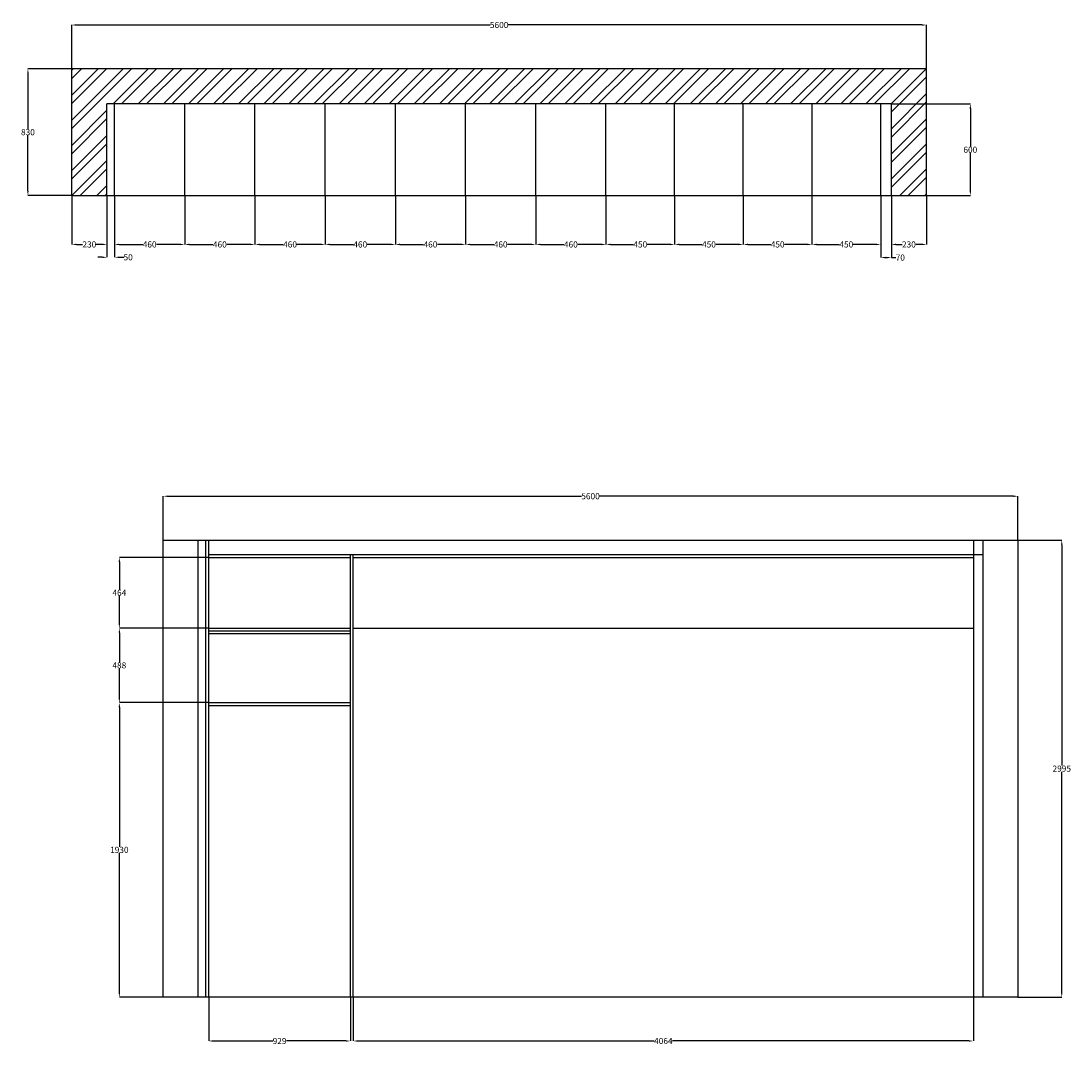
# Model space of a CAD drawing. Units: millimetres. Extents: x -17156 to 39375, y -45872 to -24892.
# Tile 12 of 12: x 32495 to 39375, y -41980 to -35270. Entities that reach past the tile are written whole.
import ezdxf

# ---------------------------------------------------------------- set-up
doc = ezdxf.new("R2010")
doc.units = ezdxf.units.MM
doc.header["$MEASUREMENT"] = 0
doc.layers.add('A-ANNO-DIMS', color=2, linetype='Continuous', lineweight=18)
doc.layers.add('A-DETL', color=7, linetype='Continuous', lineweight=25)
doc.layers.add('A-DETL-PATT', color=114, linetype='Continuous', lineweight=13, true_color=0x139b48)
doc.styles.get("Standard").update_dxf_attribs({"font": 'arial.ttf'})
doc.dimstyles.get("Standard").update_dxf_attribs({"dimtxt": 40, "dimasz": 30.18, "dimexe": 0, "dimexo": 0.0625, "dimgap": 0.09, "dimtad": 0, "dimtih": 1, "dimtoh": 1, "dimdec": 0, "dimzin": 0, "dimdsep": 46, "dimtxsty": 'Standard', "dimcen": 0.09, "dimadec": 0, "dimazin": 0, "dimtfac": 1, "dimtdec": 0, "dimtofl": 0, "dimtmove": 0, "dimatfit": 3, "dimfxl": 1, "dimtolj": 1, "dimtzin": 0, "dimarcsym": 0})

# ---------------------------------------------------------------- blocks, each defined once
blk = doc.blocks.new('*D118')
at = {"layer": 'A-ANNO-DIMS', "color": 0, "lineweight": -2, "transparency": 16777216}
for p, q in [((32827.5, -36413.8), (32827.5, -36734.2)), ((33057.5, -36413.8), (33057.5, -36734.2)), ((32857.7, -36734.2), (32898, -36734.2)), ((33027.4, -36734.2), (32987.1, -36734.2))]:
    blk.add_line(p, q, dxfattribs=at)
at = {"layer": 'A-ANNO-DIMS', "color": 0, "lineweight": 100, "transparency": 16777216}
for points in [[(32857.7, -36729.2), (32857.7, -36739.2), (32827.5, -36734.2)], [(33027.4, -36729.2), (33027.4, -36739.2), (33057.5, -36734.2)]]:
    blk.add_solid(points, dxfattribs=at)
at = {"layer": 'Defpoints', "color": 0, "lineweight": 100, "transparency": 16777216}
for p in [(32827.5, -36413.7), (33057.5, -36413.7), (33057.5, -36734.2)]:
    blk.add_point(p, dxfattribs=at)
at = {"layer": 'A-ANNO-DIMS', "color": 0, "transparency": 16777216, "insert": (32942.5, -36734.2), "char_height": 40, "attachment_point": 5}
blk.add_mtext('\\A1;230', dxfattribs=at)
blk = doc.blocks.new('*D119')
at = {"layer": 'A-ANNO-DIMS', "color": 0, "lineweight": -2, "transparency": 16777216}
for p, q in [((33057.5, -36413.8), (33057.5, -36818.4)), ((33107.5, -36413.8), (33107.5, -36818.4)), ((33027.4, -36818.4), (32997.2, -36818.4)), ((33137.7, -36818.4), (33167.9, -36818.4))]:
    blk.add_line(p, q, dxfattribs=at)
at = {"layer": 'A-ANNO-DIMS', "color": 0, "lineweight": 100, "transparency": 16777216}
for points in [[(33027.4, -36813.3), (33027.4, -36823.4), (33057.5, -36818.4)], [(33137.7, -36813.3), (33137.7, -36823.4), (33107.5, -36818.4)]]:
    blk.add_solid(points, dxfattribs=at)
at = {"layer": 'Defpoints', "color": 0, "lineweight": 100, "transparency": 16777216}
for p in [(33057.5, -36413.7), (33107.5, -36413.7), (33107.5, -36818.4)]:
    blk.add_point(p, dxfattribs=at)
at = {"layer": 'A-ANNO-DIMS', "color": 0, "transparency": 16777216, "insert": (33196.6, -36818.4), "char_height": 40, "attachment_point": 5}
blk.add_mtext('\\A1;50', dxfattribs=at)
blk = doc.blocks.new('*D120')
at = {"layer": 'A-ANNO-DIMS', "color": 0, "lineweight": -2, "transparency": 16777216}
for p, q in [((33107.5, -36413.8), (33107.5, -36734.2)), ((33567.5, -36413.8), (33567.5, -36734.2)), ((33137.7, -36734.2), (33292.5, -36734.2)), ((33537.4, -36734.2), (33382.6, -36734.2))]:
    blk.add_line(p, q, dxfattribs=at)
at = {"layer": 'A-ANNO-DIMS', "color": 0, "lineweight": 100, "transparency": 16777216}
for points in [[(33137.7, -36729.2), (33137.7, -36739.2), (33107.5, -36734.2)], [(33537.4, -36729.2), (33537.4, -36739.2), (33567.5, -36734.2)]]:
    blk.add_solid(points, dxfattribs=at)
at = {"layer": 'Defpoints', "color": 0, "lineweight": 100, "transparency": 16777216}
for p in [(33107.5, -36413.7), (33567.5, -36413.7), (33567.5, -36734.2)]:
    blk.add_point(p, dxfattribs=at)
at = {"layer": 'A-ANNO-DIMS', "color": 0, "transparency": 16777216, "insert": (33337.5, -36734.2), "char_height": 40, "attachment_point": 5}
blk.add_mtext('\\A1;460', dxfattribs=at)
blk = doc.blocks.new('*D121')
at = {"layer": 'A-ANNO-DIMS', "color": 0, "lineweight": -2, "transparency": 16777216}
for p, q in [((33567.5, -36413.8), (33567.5, -36734.2)), ((34027.5, -36413.8), (34027.5, -36734.2)), ((33597.7, -36734.2), (33752.5, -36734.2)), ((33997.4, -36734.2), (33842.6, -36734.2))]:
    blk.add_line(p, q, dxfattribs=at)
at = {"layer": 'A-ANNO-DIMS', "color": 0, "lineweight": 100, "transparency": 16777216}
for points in [[(33597.7, -36729.2), (33597.7, -36739.2), (33567.5, -36734.2)], [(33997.4, -36729.2), (33997.4, -36739.2), (34027.5, -36734.2)]]:
    blk.add_solid(points, dxfattribs=at)
at = {"layer": 'Defpoints', "color": 0, "lineweight": 100, "transparency": 16777216}
for p in [(33567.5, -36413.7), (34027.5, -36413.7), (34027.5, -36734.2)]:
    blk.add_point(p, dxfattribs=at)
at = {"layer": 'A-ANNO-DIMS', "color": 0, "transparency": 16777216, "insert": (33797.5, -36734.2), "char_height": 40, "attachment_point": 5}
blk.add_mtext('\\A1;460', dxfattribs=at)
blk = doc.blocks.new('*D122')
at = {"layer": 'A-ANNO-DIMS', "color": 0, "lineweight": -2, "transparency": 16777216}
for p, q in [((34027.5, -36413.8), (34027.5, -36734.2)), ((34487.5, -36413.8), (34487.5, -36734.2)), ((34057.7, -36734.2), (34212.5, -36734.2)), ((34457.4, -36734.2), (34302.6, -36734.2))]:
    blk.add_line(p, q, dxfattribs=at)
at = {"layer": 'A-ANNO-DIMS', "color": 0, "lineweight": 100, "transparency": 16777216}
for points in [[(34057.7, -36729.2), (34057.7, -36739.2), (34027.5, -36734.2)], [(34457.4, -36729.2), (34457.4, -36739.2), (34487.5, -36734.2)]]:
    blk.add_solid(points, dxfattribs=at)
at = {"layer": 'Defpoints', "color": 0, "lineweight": 100, "transparency": 16777216}
for p in [(34027.5, -36413.7), (34487.5, -36413.7), (34487.5, -36734.2)]:
    blk.add_point(p, dxfattribs=at)
at = {"layer": 'A-ANNO-DIMS', "color": 0, "transparency": 16777216, "insert": (34257.5, -36734.2), "char_height": 40, "attachment_point": 5}
blk.add_mtext('\\A1;460', dxfattribs=at)
blk = doc.blocks.new('*D123')
at = {"layer": 'A-ANNO-DIMS', "color": 0, "lineweight": -2, "transparency": 16777216}
for p, q in [((34487.5, -36413.8), (34487.5, -36734.2)), ((34947.5, -36413.8), (34947.5, -36734.2)), ((34517.7, -36734.2), (34672.5, -36734.2)), ((34917.4, -36734.2), (34762.6, -36734.2))]:
    blk.add_line(p, q, dxfattribs=at)
at = {"layer": 'A-ANNO-DIMS', "color": 0, "lineweight": 100, "transparency": 16777216}
for points in [[(34517.7, -36729.2), (34517.7, -36739.2), (34487.5, -36734.2)], [(34917.4, -36729.2), (34917.4, -36739.2), (34947.5, -36734.2)]]:
    blk.add_solid(points, dxfattribs=at)
at = {"layer": 'Defpoints', "color": 0, "lineweight": 100, "transparency": 16777216}
for p in [(34487.5, -36413.7), (34947.5, -36413.7), (34947.5, -36734.2)]:
    blk.add_point(p, dxfattribs=at)
at = {"layer": 'A-ANNO-DIMS', "color": 0, "transparency": 16777216, "insert": (34717.5, -36734.2), "char_height": 40, "attachment_point": 5}
blk.add_mtext('\\A1;460', dxfattribs=at)
blk = doc.blocks.new('*D124')
at = {"layer": 'A-ANNO-DIMS', "color": 0, "lineweight": -2, "transparency": 16777216}
for p, q in [((34947.5, -36413.8), (34947.5, -36734.2)), ((35407.5, -36413.8), (35407.5, -36734.2)), ((34977.7, -36734.2), (35132.5, -36734.2)), ((35377.4, -36734.2), (35222.6, -36734.2))]:
    blk.add_line(p, q, dxfattribs=at)
at = {"layer": 'A-ANNO-DIMS', "color": 0, "lineweight": 100, "transparency": 16777216}
for points in [[(34977.7, -36729.2), (34977.7, -36739.2), (34947.5, -36734.2)], [(35377.4, -36729.2), (35377.4, -36739.2), (35407.5, -36734.2)]]:
    blk.add_solid(points, dxfattribs=at)
at = {"layer": 'Defpoints', "color": 0, "lineweight": 100, "transparency": 16777216}
for p in [(34947.5, -36413.7), (35407.5, -36413.7), (35407.5, -36734.2)]:
    blk.add_point(p, dxfattribs=at)
at = {"layer": 'A-ANNO-DIMS', "color": 0, "transparency": 16777216, "insert": (35177.5, -36734.2), "char_height": 40, "attachment_point": 5}
blk.add_mtext('\\A1;460', dxfattribs=at)
blk = doc.blocks.new('*D125')
at = {"layer": 'A-ANNO-DIMS', "color": 0, "lineweight": -2, "transparency": 16777216}
for p, q in [((35407.5, -36413.8), (35407.5, -36734.2)), ((35867.5, -36413.8), (35867.5, -36734.2)), ((35437.7, -36734.2), (35592.5, -36734.2)), ((35837.4, -36734.2), (35682.6, -36734.2))]:
    blk.add_line(p, q, dxfattribs=at)
at = {"layer": 'A-ANNO-DIMS', "color": 0, "lineweight": 100, "transparency": 16777216}
for points in [[(35437.7, -36729.2), (35437.7, -36739.2), (35407.5, -36734.2)], [(35837.4, -36729.2), (35837.4, -36739.2), (35867.5, -36734.2)]]:
    blk.add_solid(points, dxfattribs=at)
at = {"layer": 'Defpoints', "color": 0, "lineweight": 100, "transparency": 16777216}
for p in [(35407.5, -36413.7), (35867.5, -36413.7), (35867.5, -36734.2)]:
    blk.add_point(p, dxfattribs=at)
at = {"layer": 'A-ANNO-DIMS', "color": 0, "transparency": 16777216, "insert": (35637.5, -36734.2), "char_height": 40, "attachment_point": 5}
blk.add_mtext('\\A1;460', dxfattribs=at)
blk = doc.blocks.new('*D126')
at = {"layer": 'A-ANNO-DIMS', "color": 0, "lineweight": -2, "transparency": 16777216}
for p, q in [((35867.5, -36413.8), (35867.5, -36734.2)), ((36327.5, -36413.8), (36327.5, -36734.2)), ((35897.7, -36734.2), (36052.5, -36734.2)), ((36297.4, -36734.2), (36142.6, -36734.2))]:
    blk.add_line(p, q, dxfattribs=at)
at = {"layer": 'A-ANNO-DIMS', "color": 0, "lineweight": 100, "transparency": 16777216}
for points in [[(35897.7, -36729.2), (35897.7, -36739.2), (35867.5, -36734.2)], [(36297.4, -36729.2), (36297.4, -36739.2), (36327.5, -36734.2)]]:
    blk.add_solid(points, dxfattribs=at)
at = {"layer": 'Defpoints', "color": 0, "lineweight": 100, "transparency": 16777216}
for p in [(35867.5, -36413.7), (36327.5, -36413.7), (36327.5, -36734.2)]:
    blk.add_point(p, dxfattribs=at)
at = {"layer": 'A-ANNO-DIMS', "color": 0, "transparency": 16777216, "insert": (36097.5, -36734.2), "char_height": 40, "attachment_point": 5}
blk.add_mtext('\\A1;460', dxfattribs=at)
blk = doc.blocks.new('*D127')
at = {"layer": 'A-ANNO-DIMS', "color": 0, "lineweight": -2, "transparency": 16777216}
for p, q in [((36327.5, -36413.8), (36327.5, -36734.2)), ((36777.5, -36413.8), (36777.5, -36734.2)), ((36357.7, -36734.2), (36507.5, -36734.2)), ((36747.4, -36734.2), (36597.6, -36734.2))]:
    blk.add_line(p, q, dxfattribs=at)
at = {"layer": 'A-ANNO-DIMS', "color": 0, "lineweight": 100, "transparency": 16777216}
for points in [[(36357.7, -36729.2), (36357.7, -36739.2), (36327.5, -36734.2)], [(36747.4, -36729.2), (36747.4, -36739.2), (36777.5, -36734.2)]]:
    blk.add_solid(points, dxfattribs=at)
at = {"layer": 'Defpoints', "color": 0, "lineweight": 100, "transparency": 16777216}
for p in [(36327.5, -36413.7), (36777.5, -36413.7), (36777.5, -36734.2)]:
    blk.add_point(p, dxfattribs=at)
at = {"layer": 'A-ANNO-DIMS', "color": 0, "transparency": 16777216, "insert": (36552.5, -36734.2), "char_height": 40, "attachment_point": 5}
blk.add_mtext('\\A1;450', dxfattribs=at)
blk = doc.blocks.new('*D128')
at = {"layer": 'A-ANNO-DIMS', "color": 0, "lineweight": -2, "transparency": 16777216}
for p, q in [((36777.5, -36413.8), (36777.5, -36734.2)), ((37227.5, -36413.8), (37227.5, -36734.2)), ((36807.7, -36734.2), (36957.5, -36734.2)), ((37197.4, -36734.2), (37047.6, -36734.2))]:
    blk.add_line(p, q, dxfattribs=at)
at = {"layer": 'A-ANNO-DIMS', "color": 0, "lineweight": 100, "transparency": 16777216}
for points in [[(36807.7, -36729.2), (36807.7, -36739.2), (36777.5, -36734.2)], [(37197.4, -36729.2), (37197.4, -36739.2), (37227.5, -36734.2)]]:
    blk.add_solid(points, dxfattribs=at)
at = {"layer": 'Defpoints', "color": 0, "lineweight": 100, "transparency": 16777216}
for p in [(36777.5, -36413.7), (37227.5, -36413.7), (37227.5, -36734.2)]:
    blk.add_point(p, dxfattribs=at)
at = {"layer": 'A-ANNO-DIMS', "color": 0, "transparency": 16777216, "insert": (37002.5, -36734.2), "char_height": 40, "attachment_point": 5}
blk.add_mtext('\\A1;450', dxfattribs=at)
blk = doc.blocks.new('*D129')
at = {"layer": 'A-ANNO-DIMS', "color": 0, "lineweight": -2, "transparency": 16777216}
for p, q in [((37227.5, -36413.8), (37227.5, -36734.2)), ((37677.5, -36413.8), (37677.5, -36734.2)), ((37257.7, -36734.2), (37407.5, -36734.2)), ((37647.4, -36734.2), (37497.6, -36734.2))]:
    blk.add_line(p, q, dxfattribs=at)
at = {"layer": 'A-ANNO-DIMS', "color": 0, "lineweight": 100, "transparency": 16777216}
for points in [[(37257.7, -36729.2), (37257.7, -36739.2), (37227.5, -36734.2)], [(37647.4, -36729.2), (37647.4, -36739.2), (37677.5, -36734.2)]]:
    blk.add_solid(points, dxfattribs=at)
at = {"layer": 'Defpoints', "color": 0, "lineweight": 100, "transparency": 16777216}
for p in [(37227.5, -36413.7), (37677.5, -36413.7), (37677.5, -36734.2)]:
    blk.add_point(p, dxfattribs=at)
at = {"layer": 'A-ANNO-DIMS', "color": 0, "transparency": 16777216, "insert": (37452.5, -36734.2), "char_height": 40, "attachment_point": 5}
blk.add_mtext('\\A1;450', dxfattribs=at)
blk = doc.blocks.new('*D130')
at = {"layer": 'A-ANNO-DIMS', "color": 0, "lineweight": -2, "transparency": 16777216}
for p, q in [((37677.5, -36413.8), (37677.5, -36734.2)), ((38127.5, -36413.8), (38127.5, -36734.2)), ((37707.7, -36734.2), (37857.5, -36734.2)), ((38097.4, -36734.2), (37947.6, -36734.2))]:
    blk.add_line(p, q, dxfattribs=at)
at = {"layer": 'A-ANNO-DIMS', "color": 0, "lineweight": 100, "transparency": 16777216}
for points in [[(37707.7, -36729.2), (37707.7, -36739.2), (37677.5, -36734.2)], [(38097.4, -36729.2), (38097.4, -36739.2), (38127.5, -36734.2)]]:
    blk.add_solid(points, dxfattribs=at)
at = {"layer": 'Defpoints', "color": 0, "lineweight": 100, "transparency": 16777216}
for p in [(37677.5, -36413.7), (38127.5, -36413.7), (38127.5, -36734.2)]:
    blk.add_point(p, dxfattribs=at)
at = {"layer": 'A-ANNO-DIMS', "color": 0, "transparency": 16777216, "insert": (37902.5, -36734.2), "char_height": 40, "attachment_point": 5}
blk.add_mtext('\\A1;450', dxfattribs=at)
blk = doc.blocks.new('*D131')
at = {"layer": 'A-ANNO-DIMS', "color": 0, "lineweight": -2, "transparency": 16777216}
for p, q in [((38127.5, -36413.8), (38127.5, -36820.2)), ((38197.5, -36413.8), (38197.5, -36820.2)), ((38157.7, -36820.2), (38167.4, -36820.2)), ((38197.5, -36820.2), (38227.7, -36820.2))]:
    blk.add_line(p, q, dxfattribs=at)
at = {"layer": 'A-ANNO-DIMS', "color": 0, "lineweight": 100, "transparency": 16777216}
for points in [[(38157.7, -36815.2), (38157.7, -36825.2), (38127.5, -36820.2)], [(38167.4, -36815.2), (38167.4, -36825.2), (38197.5, -36820.2)]]:
    blk.add_solid(points, dxfattribs=at)
at = {"layer": 'Defpoints', "color": 0, "lineweight": 100, "transparency": 16777216}
for p in [(38127.5, -36413.7), (38197.5, -36413.7), (38197.5, -36820.2)]:
    blk.add_point(p, dxfattribs=at)
at = {"layer": 'A-ANNO-DIMS', "color": 0, "transparency": 16777216, "insert": (38256.2, -36820.2), "char_height": 40, "attachment_point": 5}
blk.add_mtext('\\A1;70', dxfattribs=at)
blk = doc.blocks.new('*D132')
at = {"layer": 'A-ANNO-DIMS', "color": 0, "lineweight": -2, "transparency": 16777216}
for p, q in [((38197.5, -36413.8), (38197.5, -36734.2)), ((38427.5, -36413.8), (38427.5, -36734.2)), ((38227.7, -36734.2), (38268, -36734.2)), ((38397.4, -36734.2), (38357.1, -36734.2))]:
    blk.add_line(p, q, dxfattribs=at)
at = {"layer": 'A-ANNO-DIMS', "color": 0, "lineweight": 100, "transparency": 16777216}
for points in [[(38227.7, -36729.2), (38227.7, -36739.2), (38197.5, -36734.2)], [(38397.4, -36729.2), (38397.4, -36739.2), (38427.5, -36734.2)]]:
    blk.add_solid(points, dxfattribs=at)
at = {"layer": 'Defpoints', "color": 0, "lineweight": 100, "transparency": 16777216}
for p in [(38197.5, -36413.7), (38427.5, -36413.7), (38427.5, -36734.2)]:
    blk.add_point(p, dxfattribs=at)
at = {"layer": 'A-ANNO-DIMS', "color": 0, "transparency": 16777216, "insert": (38312.5, -36734.2), "char_height": 40, "attachment_point": 5}
blk.add_mtext('\\A1;230', dxfattribs=at)
blk = doc.blocks.new('*D154')
at = {"layer": 'A-ANNO-DIMS', "color": 0, "lineweight": -2, "transparency": 16777216}
for p, q in [((32827.5, -35583.7), (32827.5, -35296.2)), ((32857.7, -35296.2), (35567.8, -35296.2)), ((38397.4, -35296.2), (35687.3, -35296.2)), ((38427.5, -35583.7), (38427.5, -35296.2))]:
    blk.add_line(p, q, dxfattribs=at)
at = {"layer": 'A-ANNO-DIMS', "color": 0, "lineweight": 100, "transparency": 16777216}
for points in [[(32857.7, -35291.2), (32857.7, -35301.3), (32827.5, -35296.2)], [(38397.4, -35291.2), (38397.4, -35301.3), (38427.5, -35296.2)]]:
    blk.add_solid(points, dxfattribs=at)
at = {"layer": 'Defpoints', "color": 0, "lineweight": 100, "transparency": 16777216}
for p in [(38427.5, -35296.2), (32827.5, -35583.7), (38427.5, -35583.7)]:
    blk.add_point(p, dxfattribs=at)
at = {"layer": 'A-ANNO-DIMS', "color": 0, "transparency": 16777216, "insert": (35627.5, -35296.2), "char_height": 40, "attachment_point": 5}
blk.add_mtext('\\A1;5600', dxfattribs=at)
blk = doc.blocks.new('*D155')
at = {"layer": 'A-ANNO-DIMS', "color": 0, "lineweight": -2, "transparency": 16777216}
for p, q in [((32827.5, -35583.7), (32540, -35583.7)), ((32540, -35613.9), (32540, -35978.2)), ((32540, -36383.5), (32540, -36019.3)), ((32827.5, -36413.7), (32540, -36413.7))]:
    blk.add_line(p, q, dxfattribs=at)
at = {"layer": 'A-ANNO-DIMS', "color": 0, "lineweight": 100, "transparency": 16777216}
for points in [[(32535, -35613.9), (32545.1, -35613.9), (32540, -35583.7)], [(32535, -36383.5), (32545.1, -36383.5), (32540, -36413.7)]]:
    blk.add_solid(points, dxfattribs=at)
at = {"layer": 'Defpoints', "color": 0, "lineweight": 100, "transparency": 16777216}
for p in [(32827.5, -35583.7), (32540, -36413.7), (32827.5, -36413.7)]:
    blk.add_point(p, dxfattribs=at)
at = {"layer": 'A-ANNO-DIMS', "color": 0, "transparency": 16777216, "insert": (32540, -35998.7), "char_height": 40, "attachment_point": 5}
blk.add_mtext('\\A1;830', dxfattribs=at)
blk = doc.blocks.new('*D156')
at = {"layer": 'A-ANNO-DIMS', "color": 0, "lineweight": -2, "transparency": 16777216}
for p, q in [((38197.6, -35813.7), (38715, -35813.7)), ((38715, -35843.9), (38715, -36093.2)), ((38715, -36383.5), (38715, -36134.2)), ((38197.6, -36413.7), (38715, -36413.7))]:
    blk.add_line(p, q, dxfattribs=at)
at = {"layer": 'A-ANNO-DIMS', "color": 0, "lineweight": 100, "transparency": 16777216}
for points in [[(38710, -35843.9), (38720.1, -35843.9), (38715, -35813.7)], [(38710, -36383.5), (38720.1, -36383.5), (38715, -36413.7)]]:
    blk.add_solid(points, dxfattribs=at)
at = {"layer": 'Defpoints', "color": 0, "lineweight": 100, "transparency": 16777216}
for p in [(38197.5, -35813.7), (38197.5, -36413.7), (38715, -36413.7)]:
    blk.add_point(p, dxfattribs=at)
at = {"layer": 'A-ANNO-DIMS', "color": 0, "transparency": 16777216, "insert": (38715, -36113.7), "char_height": 40, "attachment_point": 5}
blk.add_mtext('\\A1;600', dxfattribs=at)
blk = doc.blocks.new('*D157')
at = {"layer": 'A-ANNO-DIMS', "color": 0, "lineweight": -2, "transparency": 16777216}
for p, q in [((33426.5, -38671.7), (33426.5, -38384.2)), ((33456.7, -38384.2), (36166.7, -38384.2)), ((38996.3, -38384.2), (36286.2, -38384.2)), ((39026.5, -38671.7), (39026.5, -38384.2))]:
    blk.add_line(p, q, dxfattribs=at)
at = {"layer": 'A-ANNO-DIMS', "color": 0, "lineweight": 100, "transparency": 16777216}
for points in [[(33456.7, -38379.2), (33456.7, -38389.2), (33426.5, -38384.2)], [(38996.3, -38379.2), (38996.3, -38389.2), (39026.5, -38384.2)]]:
    blk.add_solid(points, dxfattribs=at)
at = {"layer": 'Defpoints', "color": 0, "lineweight": 100, "transparency": 16777216}
for p in [(39026.5, -38384.2), (33426.5, -38671.7), (39026.5, -38671.7)]:
    blk.add_point(p, dxfattribs=at)
at = {"layer": 'A-ANNO-DIMS', "color": 0, "transparency": 16777216, "insert": (36226.5, -38384.2), "char_height": 40, "attachment_point": 5}
blk.add_mtext('\\A1;5600', dxfattribs=at)
blk = doc.blocks.new('*D158')
at = {"layer": 'A-ANNO-DIMS', "color": 0, "lineweight": -2, "transparency": 16777216}
for p, q in [((39026.6, -38671.7), (39314, -38671.7)), ((39314, -38701.9), (39314, -40148.7)), ((39314, -41636.5), (39314, -40189.7)), ((39026.6, -41666.7), (39314, -41666.7))]:
    blk.add_line(p, q, dxfattribs=at)
at = {"layer": 'A-ANNO-DIMS', "color": 0, "lineweight": 100, "transparency": 16777216}
for points in [[(39309, -38701.9), (39319, -38701.9), (39314, -38671.7)], [(39309, -41636.5), (39319, -41636.5), (39314, -41666.7)]]:
    blk.add_solid(points, dxfattribs=at)
at = {"layer": 'Defpoints', "color": 0, "lineweight": 100, "transparency": 16777216}
for p in [(39026.5, -38671.7), (39314, -38671.7), (39026.5, -41666.7)]:
    blk.add_point(p, dxfattribs=at)
at = {"layer": 'A-ANNO-DIMS', "color": 0, "transparency": 16777216, "insert": (39314, -40169.2), "char_height": 40, "attachment_point": 5}
blk.add_mtext('\\A1;2995', dxfattribs=at)
blk = doc.blocks.new('*D159')
at = {"layer": 'A-ANNO-DIMS', "color": 0, "lineweight": -2, "transparency": 16777216}
for p, q in [((33724.5, -41666.8), (33724.5, -41954.2)), ((34653.5, -41666.8), (34653.5, -41954.2)), ((33754.7, -41954.2), (34144.7, -41954.2)), ((34623.3, -41954.2), (34233.3, -41954.2))]:
    blk.add_line(p, q, dxfattribs=at)
at = {"layer": 'A-ANNO-DIMS', "color": 0, "lineweight": 100, "transparency": 16777216}
for points in [[(33754.7, -41949.2), (33754.7, -41959.2), (33724.5, -41954.2)], [(34623.3, -41949.2), (34623.3, -41959.2), (34653.5, -41954.2)]]:
    blk.add_solid(points, dxfattribs=at)
at = {"layer": 'Defpoints', "color": 0, "lineweight": 100, "transparency": 16777216}
for p in [(33724.5, -41666.7), (34653.5, -41666.7), (34653.5, -41954.2)]:
    blk.add_point(p, dxfattribs=at)
at = {"layer": 'A-ANNO-DIMS', "color": 0, "transparency": 16777216, "insert": (34189, -41954.2), "char_height": 40, "attachment_point": 5}
blk.add_mtext('\\A1;929', dxfattribs=at)
blk = doc.blocks.new('*D160')
at = {"layer": 'A-ANNO-DIMS', "color": 0, "lineweight": -2, "transparency": 16777216}
for p, q in [((34671.5, -41666.8), (34671.5, -41954.2)), ((38735.5, -41666.8), (38735.5, -41954.2)), ((34701.7, -41954.2), (36643, -41954.2)), ((38705.3, -41954.2), (36764, -41954.2))]:
    blk.add_line(p, q, dxfattribs=at)
at = {"layer": 'A-ANNO-DIMS', "color": 0, "lineweight": 100, "transparency": 16777216}
for points in [[(34701.7, -41949.2), (34701.7, -41959.2), (34671.5, -41954.2)], [(38705.3, -41949.2), (38705.3, -41959.2), (38735.5, -41954.2)]]:
    blk.add_solid(points, dxfattribs=at)
at = {"layer": 'Defpoints', "color": 0, "lineweight": 100, "transparency": 16777216}
for p in [(34671.5, -41666.7), (38735.5, -41666.7), (38735.5, -41954.2)]:
    blk.add_point(p, dxfattribs=at)
at = {"layer": 'A-ANNO-DIMS', "color": 0, "transparency": 16777216, "insert": (36703.5, -41954.2), "char_height": 40, "attachment_point": 5}
blk.add_mtext('\\A1;4064', dxfattribs=at)
blk = doc.blocks.new('*D161')
at = {"layer": 'A-ANNO-DIMS', "color": 0, "lineweight": -2, "transparency": 16777216}
for p, q in [((33724.4, -39736.7), (33139, -39736.7)), ((33139, -39766.9), (33139, -40681.2)), ((33139, -41636.5), (33139, -40722.2)), ((33724.4, -41666.7), (33139, -41666.7))]:
    blk.add_line(p, q, dxfattribs=at)
at = {"layer": 'A-ANNO-DIMS', "color": 0, "lineweight": 100, "transparency": 16777216}
for points in [[(33134, -39766.9), (33144, -39766.9), (33139, -39736.7)], [(33134, -41636.5), (33144, -41636.5), (33139, -41666.7)]]:
    blk.add_solid(points, dxfattribs=at)
at = {"layer": 'Defpoints', "color": 0, "lineweight": 100, "transparency": 16777216}
for p in [(33139, -39736.7), (33724.5, -39736.7), (33724.5, -41666.7)]:
    blk.add_point(p, dxfattribs=at)
at = {"layer": 'A-ANNO-DIMS', "color": 0, "transparency": 16777216, "insert": (33139, -40701.7), "char_height": 40, "attachment_point": 5}
blk.add_mtext('\\A1;1930', dxfattribs=at)
blk = doc.blocks.new('*D162')
at = {"layer": 'A-ANNO-DIMS', "color": 0, "lineweight": -2, "transparency": 16777216}
for p, q in [((33724.4, -39248.7), (33139, -39248.7)), ((33139, -39278.9), (33139, -39472.2)), ((33139, -39706.5), (33139, -39513.2)), ((33724.4, -39736.7), (33139, -39736.7))]:
    blk.add_line(p, q, dxfattribs=at)
at = {"layer": 'A-ANNO-DIMS', "color": 0, "lineweight": 100, "transparency": 16777216}
for points in [[(33134, -39278.9), (33144, -39278.9), (33139, -39248.7)], [(33134, -39706.5), (33144, -39706.5), (33139, -39736.7)]]:
    blk.add_solid(points, dxfattribs=at)
at = {"layer": 'Defpoints', "color": 0, "lineweight": 100, "transparency": 16777216}
for p in [(33139, -39248.7), (33724.5, -39248.7), (33724.5, -39736.7)]:
    blk.add_point(p, dxfattribs=at)
at = {"layer": 'A-ANNO-DIMS', "color": 0, "transparency": 16777216, "insert": (33139, -39492.7), "char_height": 40, "attachment_point": 5}
blk.add_mtext('\\A1;488', dxfattribs=at)
blk = doc.blocks.new('*D163')
at = {"layer": 'A-ANNO-DIMS', "color": 0, "lineweight": -2, "transparency": 16777216}
for p, q in [((33724.4, -38784.7), (33139, -38784.7)), ((33139, -38814.9), (33139, -38996.2)), ((33139, -39218.5), (33139, -39037.2)), ((33724.4, -39248.7), (33139, -39248.7))]:
    blk.add_line(p, q, dxfattribs=at)
at = {"layer": 'A-ANNO-DIMS', "color": 0, "lineweight": 100, "transparency": 16777216}
for points in [[(33134, -38814.9), (33144, -38814.9), (33139, -38784.7)], [(33134, -39218.5), (33144, -39218.5), (33139, -39248.7)]]:
    blk.add_solid(points, dxfattribs=at)
at = {"layer": 'Defpoints', "color": 0, "lineweight": 100, "transparency": 16777216}
for p in [(33139, -38784.7), (33724.5, -38784.7), (33724.5, -39248.7)]:
    blk.add_point(p, dxfattribs=at)
at = {"layer": 'A-ANNO-DIMS', "color": 0, "transparency": 16777216, "insert": (33139, -39016.7), "char_height": 40, "attachment_point": 5}
blk.add_mtext('\\A1;464', dxfattribs=at)

msp = doc.modelspace()

# ---------------------------------------------------------------- hatches: boundary and pattern name
at = {"layer": 'A-DETL-PATT'}
h = msp.add_hatch(dxfattribs=at)
h.set_pattern_fill('ANSI32', color=256, scale=310)
h.set_pattern_definition([(45, (32827.54, -36413.73), (-82.2012, 82.2012), []), (45, (32882.34, -36413.73), (-82.2012, 82.2012), [])])
h.paths.add_polyline_path([(38427.54, -35583.73), (32827.54, -35583.73), (32827.54, -35813.73), (32827.54, -36413.73), (33057.54, -36413.73), (33057.54, -35813.73), (38197.54, -35813.73), (38197.54, -36413.73), (38427.54, -36413.73), (38427.54, -35813.73)])

# ---------------------------------------------------------------- linework, layer by layer
at = {"layer": 'A-DETL'}
for p, q in [((32827.54, -35813.73), (32827.54, -35583.73)), ((38427.54, -35583.73), (32827.54, -35583.73)), ((38427.54, -35813.73), (38427.54, -35583.73)), ((32827.54, -36413.73), (32827.54, -35813.73)), ((33057.54, -36413.73), (33057.54, -35813.73)), ((38197.54, -35813.73), (33057.54, -35813.73)), ((33107.54, -36413.73), (33107.54, -35813.73)), ((33567.54, -36413.73), (33567.54, -35813.73)), ((34027.54, -36413.73), (34027.54, -35813.73)), ((34487.54, -36413.73), (34487.54, -35813.73)), ((34947.54, -36413.73), (34947.54, -35813.73)), ((35407.54, -36413.73), (35407.54, -35813.73)), ((35867.54, -36413.73), (35867.54, -35813.73)), ((36327.54, -36413.73), (36327.54, -35813.73)), ((36777.54, -36413.73), (36777.54, -35813.73)), ((37227.54, -36413.73), (37227.54, -35813.73)), ((37677.54, -36413.73), (37677.54, -35813.73)), ((38127.54, -36413.73), (38127.54, -35813.73)), ((38197.54, -36413.73), (38197.54, -35813.73)), ((38427.54, -36413.73), (38427.54, -35813.73)), ((32827.54, -36413.73), (38427.54, -36413.73)), ((33426.5, -41666.72), (33426.5, -38671.72)), ((33426.5, -38671.72), (33656.5, -38671.72)), ((33656.5, -41666.72), (33656.5, -38671.72)), ((33656.5, -38671.72), (38796.5, -38671.72)), ((33706.5, -41666.72), (33706.5, -38671.72)), ((33724.5, -41666.72), (33724.5, -38671.72)), ((38735.5, -38671.72), (38735.5, -41666.72)), ((38796.5, -38671.72), (39026.5, -38671.72)), ((38796.5, -38671.72), (38796.5, -41666.72)), ((39026.5, -38671.72), (39026.5, -41666.72)), ((33724.5, -38766.72), (38796.5, -38766.72)), ((33724.5, -38784.72), (34653.5, -38784.72)), ((34653.5, -41666.72), (34653.5, -38766.72)), ((34671.5, -41666.72), (34671.5, -38766.72)), ((34671.5, -38784.72), (38735.5, -38784.72)), ((33724.5, -39248.72), (34653.5, -39248.72)), ((33724.5, -39266.72), (34653.5, -39266.72)), ((34671.5, -39248.72), (38735.5, -39248.72)), ((33724.5, -39284.72), (34653.5, -39284.72)), ((33724.5, -39736.72), (34653.5, -39736.72)), ((33724.5, -39754.72), (34653.5, -39754.72)), ((33656.5, -41666.72), (33426.5, -41666.72)), ((38796.5, -41666.72), (33656.5, -41666.72)), ((39026.5, -41666.72), (38796.5, -41666.72))]:
    msp.add_line(p, q, dxfattribs=at)

# ---------------------------------------------------------------- dimensions: what is measured, and where the dimension line sits
at = {"layer": 'A-ANNO-DIMS'}
for base, p1, p2, override, picture, middle in [((38427.54, -35296.23), (32827.54, -35583.73), (38427.54, -35583.73), {"dimdec": 0, "dimlfac": 1, "dimrnd": 0, "dimzin": 0, "dimdsep": 46, "dimlunit": 2}, '*D154', (35627.54, -35296.23)), ((33057.54, -36734.18), (32827.54, -36413.73), (33057.54, -36413.73), {"dimclrd": 0, "dimclre": 0, "dimclrt": 0}, '*D118', (32942.54, -36734.18)), ((33107.54, -36818.37), (33057.54, -36413.73), (33107.54, -36413.73), {"dimclrd": 0, "dimclre": 0, "dimclrt": 0}, '*D119', (33196.57, -36818.37)), ((33567.54, -36734.18), (33107.54, -36413.73), (33567.54, -36413.73), {"dimclrd": 0, "dimclre": 0, "dimclrt": 0}, '*D120', (33337.54, -36734.18)), ((34027.54, -36734.18), (33567.54, -36413.73), (34027.54, -36413.73), {"dimclrd": 0, "dimclre": 0, "dimclrt": 0}, '*D121', (33797.54, -36734.18)), ((34487.54, -36734.18), (34027.54, -36413.73), (34487.54, -36413.73), {"dimclrd": 0, "dimclre": 0, "dimclrt": 0}, '*D122', (34257.54, -36734.18)), ((34947.54, -36734.18), (34487.54, -36413.73), (34947.54, -36413.73), {"dimclrd": 0, "dimclre": 0, "dimclrt": 0}, '*D123', (34717.54, -36734.18)), ((35407.54, -36734.18), (34947.54, -36413.73), (35407.54, -36413.73), {"dimclrd": 0, "dimclre": 0, "dimclrt": 0}, '*D124', (35177.54, -36734.18)), ((35867.54, -36734.18), (35407.54, -36413.73), (35867.54, -36413.73), {"dimclrd": 0, "dimclre": 0, "dimclrt": 0}, '*D125', (35637.54, -36734.18)), ((36327.54, -36734.18), (35867.54, -36413.73), (36327.54, -36413.73), {"dimclrd": 0, "dimclre": 0, "dimclrt": 0}, '*D126', (36097.54, -36734.18)), ((36777.54, -36734.18), (36327.54, -36413.73), (36777.54, -36413.73), {"dimclrd": 0, "dimclre": 0, "dimclrt": 0}, '*D127', (36552.54, -36734.18)), ((37227.54, -36734.18), (36777.54, -36413.73), (37227.54, -36413.73), {"dimclrd": 0, "dimclre": 0, "dimclrt": 0}, '*D128', (37002.54, -36734.18)), ((37677.54, -36734.18), (37227.54, -36413.73), (37677.54, -36413.73), {"dimclrd": 0, "dimclre": 0, "dimclrt": 0}, '*D129', (37452.54, -36734.18)), ((38127.54, -36734.18), (37677.54, -36413.73), (38127.54, -36413.73), {"dimclrd": 0, "dimclre": 0, "dimclrt": 0}, '*D130', (37902.54, -36734.18)), ((38197.54, -36820.19), (38127.54, -36413.73), (38197.54, -36413.73), {"dimclrd": 0, "dimclre": 0, "dimclrt": 0}, '*D131', (38256.22, -36820.19)), ((38427.54, -36734.18), (38197.54, -36413.73), (38427.54, -36413.73), {"dimclrd": 0, "dimclre": 0, "dimclrt": 0}, '*D132', (38312.54, -36734.18)), ((39026.5, -38384.22), (33426.5, -38671.72), (39026.5, -38671.72), {"dimdec": 0, "dimlfac": 1, "dimrnd": 0, "dimzin": 0, "dimdsep": 46, "dimlunit": 2}, '*D157', (36226.5, -38384.22)), ((34653.5, -41954.22), (33724.5, -41666.72), (34653.5, -41666.72), {"dimdec": 0, "dimlfac": 1, "dimrnd": 0, "dimzin": 0, "dimdsep": 46, "dimlunit": 2}, '*D159', (34189, -41954.22)), ((38735.5, -41954.22), (34671.5, -41666.72), (38735.5, -41666.72), {"dimdec": 0, "dimlfac": 1, "dimrnd": 0, "dimzin": 0, "dimdsep": 46, "dimlunit": 2}, '*D160', (36703.5, -41954.22))]:
    dim = msp.add_linear_dim(base=base, p1=p1, p2=p2, dimstyle='Standard', override=override, dxfattribs=at)
    dim.commit()
    dim.dimension.update_dxf_attribs({"geometry": picture, "text_midpoint": middle})
for base, p1, p2, picture, middle in [((32540.04, -36413.73), (32827.54, -35583.73), (32827.54, -36413.73), '*D155', (32540.04, -35998.73)), ((38715.04, -36413.73), (38197.54, -35813.73), (38197.54, -36413.73), '*D156', (38715.04, -36113.73)), ((39314, -38671.72), (39026.5, -41666.72), (39026.5, -38671.72), '*D158', (39314, -40169.22)), ((33139, -38784.72), (33724.5, -39248.72), (33724.5, -38784.72), '*D163', (33139, -39016.72)), ((33139, -39248.72), (33724.5, -39736.72), (33724.5, -39248.72), '*D162', (33139, -39492.72)), ((33139, -39736.72), (33724.5, -41666.72), (33724.5, -39736.72), '*D161', (33139, -40701.72))]:
    dim = msp.add_linear_dim(base=base, p1=p1, p2=p2, angle=90, dimstyle='Standard', override={"dimdec": 0, "dimlfac": 1, "dimrnd": 0, "dimzin": 0, "dimdsep": 46, "dimlunit": 2}, dxfattribs=at)
    dim.commit()
    dim.dimension.update_dxf_attribs({"geometry": picture, "text_midpoint": middle})

doc.saveas('drawing.dxf')
